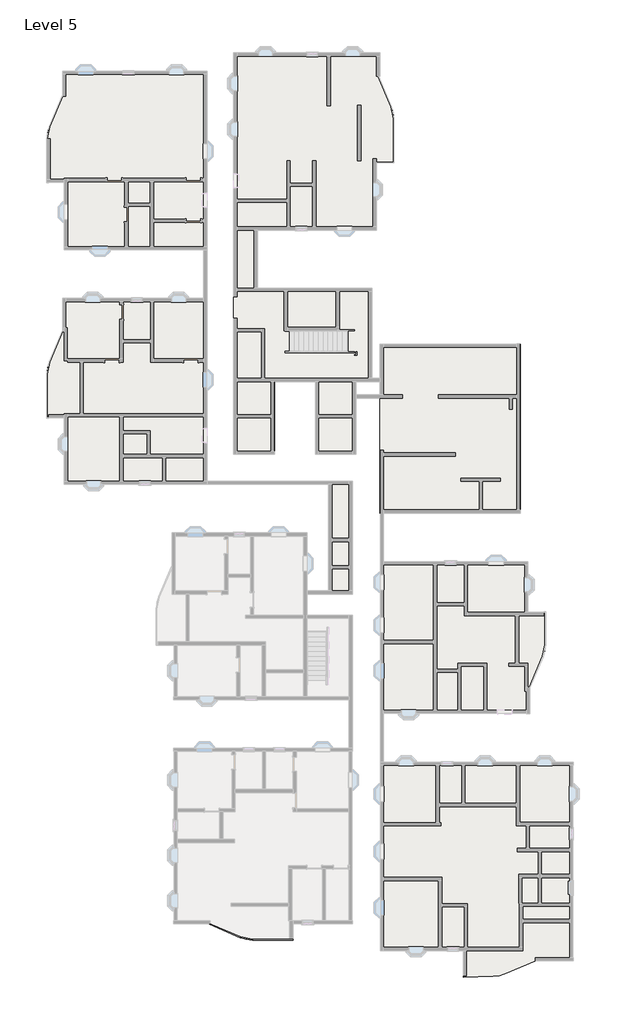
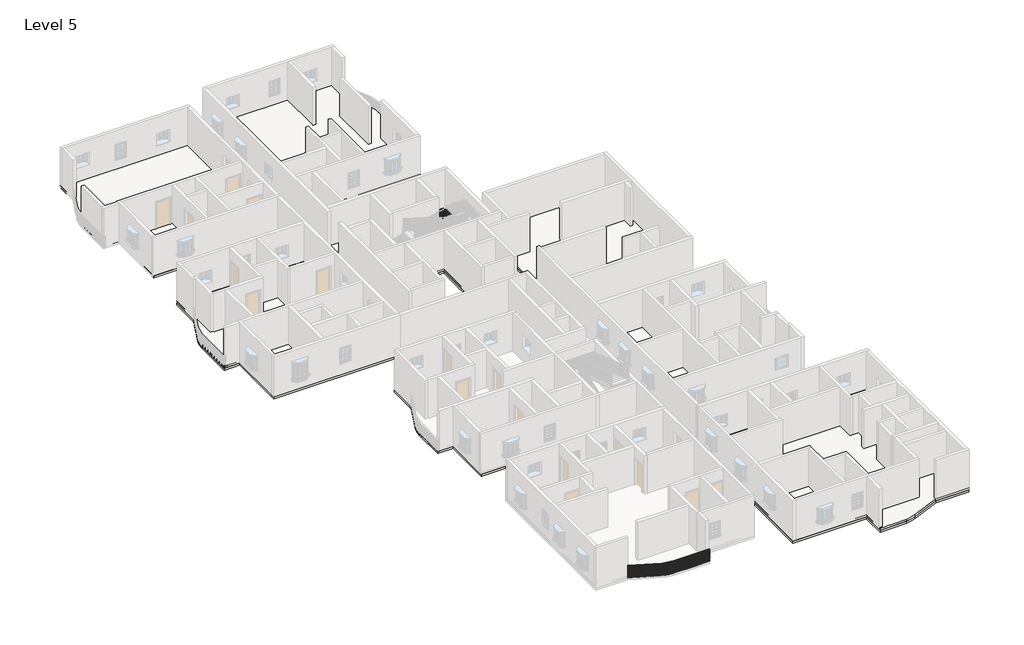
# One storey, part 5 of 14: 11 roofs, 10 slabs, 1 railing.
"""IFC4 building model written with IfcOpenShell, lengths in millimetres."""

from ifc_helpers import new_model, si_unit, point, frame, frame_2d, origin, place, context, project, spatial, polyline, circle_curve, trimmed, segment, composite_curve, outline, extrude, element, save
from ifc_brep_helpers import plane_surface, cylinder_surface, revolved_surface, advanced_brep

model = new_model("IFC4")

# Units and contexts
model_context = context("Model", 3, world=origin())
ifc_project = project(units=[si_unit("LENGTHUNIT", "METRE", prefix="MILLI")], contexts=[model_context])

# Site, building, storey
site = spatial("IfcSite", under=ifc_project)
building = spatial("IfcBuilding", under=site)
storey = spatial("IfcBuildingStorey", under=building, Name="Level 5", Elevation=12192.0)

# Railing
placement = place(None, origin())
element("IfcRailing", 1, ObjectType="Handrail - Rectangular", at=placement, inside=storey, context=model_context, shape_type="SolidModel", body=[
    advanced_brep(
    [(-10014.8722294, -25076.9923935, 13106.4), (-10014.8722294, -25076.9923935, 13055.6), (-10034.8694485, -25123.6909077, 13055.6), (-10034.8694485, -25123.6909077, 13106.4), (-8065.5370278, -25911.7359335, 13106.4), (-8065.5370278, -25911.7359335, 13055.6), (-8085.5342469, -25958.4344477, 13055.6), (-8085.5342469, -25958.4344477, 13106.4), (-7315.6413127, -26065.5416506, 13055.6), (-7315.6413127, -26065.5416506, 13106.4), (-7315.6413127, -26116.3416506, 13055.6), (-7315.6413127, -26116.3416506, 13106.4), (-4746.0891351, -26065.5416506, 13106.4), (-4746.0891351, -26116.3416506, 13106.4), (-4746.0891351, -26116.3416506, 13055.6), (-4746.0891351, -26065.5416506, 13055.6)],
    [
        (0, 1),
        (1, 2),
        (2, 3),
        (3, 0),
        (0, 4),
        (4, 5),
        (5, 1),
        (5, 6),
        (6, 2),
        (6, 7),
        (7, 3),
        (7, 4),
        (8, 5, circle_curve(frame((-7315.6413127, -24160.5416506, 13055.6), z_axis=(0.0, 0.0, -1.0), x_axis=(-0.3936460446736572, -0.9192620907623599, 0.0)), 1905.0)),
        (4, 9, circle_curve(frame((-7315.6413127, -24160.5416506, 13106.4), z_axis=(0.0, 0.0, 1.0), x_axis=(-0.3936460446736572, -0.9192620907623599, 0.0)), 1905.0)),
        (9, 8),
        (10, 6, circle_curve(frame((-7315.6413127, -24160.5416506, 13055.6), z_axis=(0.0, 0.0, -1.0), x_axis=(-0.3936460446736572, -0.9192620907623599, 0.0)), 1955.8)),
        (8, 10),
        (11, 7, circle_curve(frame((-7315.6413127, -24160.5416506, 13106.4), z_axis=(0.0, 0.0, -1.0), x_axis=(-0.3936460446736572, -0.9192620907623599, 0.0)), 1955.8)),
        (10, 11),
        (11, 9),
        (12, 13),
        (13, 14),
        (14, 15),
        (15, 12),
        (9, 12),
        (15, 8),
        (14, 10),
        (13, 11),
    ],
    [
        plane_surface(frame((-10024.8708389, -25100.3416506, 13106.4), z_axis=(-0.9192620907623597, 0.39364604467365766, 0.0), x_axis=(0.39364604467365766, 0.9192620907623597, 0.0))),
        plane_surface(frame((-10014.8722294, -25076.9923935, 13106.4), z_axis=(0.3936460446736573, 0.9192620907623599, 0.0), x_axis=(0.9192620907623599, -0.3936460446736573, 0.0))),
        plane_surface(frame((-10014.8722294, -25076.9923935, 13055.6), z_axis=(0.0, 0.0, -1.0000000000000002), x_axis=(0.9192620907623599, -0.3936460446736573, 0.0))),
        plane_surface(frame((-10034.8694485, -25123.6909077, 13055.6), z_axis=(-0.39364604467365766, -0.9192620907623597, 0.0), x_axis=(0.9192620907623597, -0.39364604467365766, 0.0))),
        plane_surface(frame((-10034.8694485, -25123.6909077, 13106.4), z_axis=(0.0, 0.0, 1.0), x_axis=(0.9192620907623597, -0.39364604467365766, 0.0))),
        revolved_surface(polyline([(-8065.537027803317, -25911.735933502296, 13106.4), (-8065.537027803317, -25911.735933502296, 13055.6)]), (-7315.6413127, -24160.5416506, 13106.4), (0.0, 0.0, 1.0)),
        plane_surface(frame((-7315.6413127, -24160.5416506, 13055.6), z_axis=(0.0, 0.0, -1.0), x_axis=(-0.3936460446736572, -0.9192620907623599, 0.0))),
        cylinder_surface(frame((-7315.6413127, -24160.5416506, 13106.4), z_axis=(0.0, 0.0, 1.0), x_axis=(-0.3936460446736572, -0.9192620907623599, 0.0)), 1955.8),
        plane_surface(frame((-7315.6413127, -24160.5416506, 13106.4), z_axis=(0.0, 0.0, 1.0), x_axis=(-0.3936460446736572, -0.9192620907623599, 0.0))),
        plane_surface(frame((-4746.0891351, -26090.9416506, 13106.4), z_axis=(1.0, 0.0, 0.0), x_axis=(0.0, 1.0, 0.0))),
        plane_surface(frame((-7315.6413127, -26065.5416506, 13106.4), z_axis=(0.0, 1.0, 0.0), x_axis=(1.0, 0.0, 0.0))),
        plane_surface(frame((-7315.6413127, -26065.5416506, 13055.6), z_axis=(0.0, 0.0, -1.0), x_axis=(1.0, 0.0, 0.0))),
        plane_surface(frame((-7315.6413127, -26116.3416506, 13055.6), z_axis=(0.0, -1.0, 0.0), x_axis=(1.0, 0.0, 0.0))),
        plane_surface(frame((-7315.6413127, -26116.3416506, 13106.4), z_axis=(0.0, 0.0, 1.0), x_axis=(1.0, 0.0, 0.0))),
    ],
    [
        (0, [[1, 2, 3, 4]]),
        (1, [[-1, 5, 6, 7]]),
        (2, [[-2, -7, 8, 9]]),
        (3, [[-3, -9, 10, 11]]),
        (4, [[-4, -11, 12, -5]]),
        (5, [[13, -6, 14, 15]]),
        (6, [[16, -8, -13, 17]]),
        (7, [[18, -10, -16, 19]]),
        (8, [[-14, -12, -18, 20]]),
        (9, [[21, 22, 23, 24]]),
        (10, [[-15, 25, -24, 26]]),
        (11, [[-17, -26, -23, 27]]),
        (12, [[-19, -27, -22, 28]]),
        (13, [[-20, -28, -21, -25]]),
    ],
),
    extrude(outline(polyline([(-4785.1663127, -26100.4666506), (-4785.1663127, -26081.4166506), (-4766.1163127, -26081.4166506), (-4766.1163127, -26100.4666506), (-4785.1663127, -26100.4666506)])), frame((0.0, 0.0, 12192.0), z_axis=(0.0, 0.0, 1.0), x_axis=(1.0, 0.0, 0.0)), (0.0, 0.0, 1.0), 863.6),
    extrude(outline(polyline([(-4886.7663127, -26100.4666506), (-4886.7663127, -26081.4166506), (-4867.7163127, -26081.4166506), (-4867.7163127, -26100.4666506), (-4886.7663127, -26100.4666506)])), frame((0.0, 0.0, 12192.0), z_axis=(0.0, 0.0, 1.0), x_axis=(1.0, 0.0, 0.0)), (0.0, 0.0, 1.0), 863.6),
    extrude(outline(polyline([(-4988.3663127, -26100.4666506), (-4988.3663127, -26081.4166506), (-4969.3163127, -26081.4166506), (-4969.3163127, -26100.4666506), (-4988.3663127, -26100.4666506)])), frame((0.0, 0.0, 12192.0), z_axis=(0.0, 0.0, 1.0), x_axis=(1.0, 0.0, 0.0)), (0.0, 0.0, 1.0), 863.6),
    extrude(outline(polyline([(-5089.9663127, -26100.4666506), (-5089.9663127, -26081.4166506), (-5070.9163127, -26081.4166506), (-5070.9163127, -26100.4666506), (-5089.9663127, -26100.4666506)])), frame((0.0, 0.0, 12192.0), z_axis=(0.0, 0.0, 1.0), x_axis=(1.0, 0.0, 0.0)), (0.0, 0.0, 1.0), 863.6),
    extrude(outline(polyline([(-5191.5663127, -26100.4666506), (-5191.5663127, -26081.4166506), (-5172.5163127, -26081.4166506), (-5172.5163127, -26100.4666506), (-5191.5663127, -26100.4666506)])), frame((0.0, 0.0, 12192.0), z_axis=(0.0, 0.0, 1.0), x_axis=(1.0, 0.0, 0.0)), (0.0, 0.0, 1.0), 863.6),
    extrude(outline(polyline([(-5293.1663127, -26100.4666506), (-5293.1663127, -26081.4166506), (-5274.1163127, -26081.4166506), (-5274.1163127, -26100.4666506), (-5293.1663127, -26100.4666506)])), frame((0.0, 0.0, 12192.0), z_axis=(0.0, 0.0, 1.0), x_axis=(1.0, 0.0, 0.0)), (0.0, 0.0, 1.0), 863.6),
    extrude(outline(polyline([(-5394.7663127, -26100.4666506), (-5394.7663127, -26081.4166506), (-5375.7163127, -26081.4166506), (-5375.7163127, -26100.4666506), (-5394.7663127, -26100.4666506)])), frame((0.0, 0.0, 12192.0), z_axis=(0.0, 0.0, 1.0), x_axis=(1.0, 0.0, 0.0)), (0.0, 0.0, 1.0), 863.6),
    extrude(outline(polyline([(-5496.3663127, -26100.4666506), (-5496.3663127, -26081.4166506), (-5477.3163127, -26081.4166506), (-5477.3163127, -26100.4666506), (-5496.3663127, -26100.4666506)])), frame((0.0, 0.0, 12192.0), z_axis=(0.0, 0.0, 1.0), x_axis=(1.0, 0.0, 0.0)), (0.0, 0.0, 1.0), 863.6),
    extrude(outline(polyline([(-5597.9663127, -26100.4666506), (-5597.9663127, -26081.4166506), (-5578.9163127, -26081.4166506), (-5578.9163127, -26100.4666506), (-5597.9663127, -26100.4666506)])), frame((0.0, 0.0, 12192.0), z_axis=(0.0, 0.0, 1.0), x_axis=(1.0, 0.0, 0.0)), (0.0, 0.0, 1.0), 863.6),
    extrude(outline(polyline([(-5699.5663127, -26100.4666506), (-5699.5663127, -26081.4166506), (-5680.5163127, -26081.4166506), (-5680.5163127, -26100.4666506), (-5699.5663127, -26100.4666506)])), frame((0.0, 0.0, 12192.0), z_axis=(0.0, 0.0, 1.0), x_axis=(1.0, 0.0, 0.0)), (0.0, 0.0, 1.0), 863.6),
    extrude(outline(polyline([(-5801.1663127, -26100.4666506), (-5801.1663127, -26081.4166506), (-5782.1163127, -26081.4166506), (-5782.1163127, -26100.4666506), (-5801.1663127, -26100.4666506)])), frame((0.0, 0.0, 12192.0), z_axis=(0.0, 0.0, 1.0), x_axis=(1.0, 0.0, 0.0)), (0.0, 0.0, 1.0), 863.6),
    extrude(outline(polyline([(-5902.7663127, -26100.4666506), (-5902.7663127, -26081.4166506), (-5883.7163127, -26081.4166506), (-5883.7163127, -26100.4666506), (-5902.7663127, -26100.4666506)])), frame((0.0, 0.0, 12192.0), z_axis=(0.0, 0.0, 1.0), x_axis=(1.0, 0.0, 0.0)), (0.0, 0.0, 1.0), 863.6),
    extrude(outline(polyline([(-6004.3663127, -26100.4666506), (-6004.3663127, -26081.4166506), (-5985.3163127, -26081.4166506), (-5985.3163127, -26100.4666506), (-6004.3663127, -26100.4666506)])), frame((0.0, 0.0, 12192.0), z_axis=(0.0, 0.0, 1.0), x_axis=(1.0, 0.0, 0.0)), (0.0, 0.0, 1.0), 863.6),
    extrude(outline(polyline([(-6105.9663127, -26100.4666506), (-6105.9663127, -26081.4166506), (-6086.9163127, -26081.4166506), (-6086.9163127, -26100.4666506), (-6105.9663127, -26100.4666506)])), frame((0.0, 0.0, 12192.0), z_axis=(0.0, 0.0, 1.0), x_axis=(1.0, 0.0, 0.0)), (0.0, 0.0, 1.0), 863.6),
    extrude(outline(polyline([(-6207.5663127, -26100.4666506), (-6207.5663127, -26081.4166506), (-6188.5163127, -26081.4166506), (-6188.5163127, -26100.4666506), (-6207.5663127, -26100.4666506)])), frame((0.0, 0.0, 12192.0), z_axis=(0.0, 0.0, 1.0), x_axis=(1.0, 0.0, 0.0)), (0.0, 0.0, 1.0), 863.6),
    extrude(outline(polyline([(-6309.1663127, -26100.4666506), (-6309.1663127, -26081.4166506), (-6290.1163127, -26081.4166506), (-6290.1163127, -26100.4666506), (-6309.1663127, -26100.4666506)])), frame((0.0, 0.0, 12192.0), z_axis=(0.0, 0.0, 1.0), x_axis=(1.0, 0.0, 0.0)), (0.0, 0.0, 1.0), 863.6),
    extrude(outline(polyline([(-6410.7663127, -26100.4666506), (-6410.7663127, -26081.4166506), (-6391.7163127, -26081.4166506), (-6391.7163127, -26100.4666506), (-6410.7663127, -26100.4666506)])), frame((0.0, 0.0, 12192.0), z_axis=(0.0, 0.0, 1.0), x_axis=(1.0, 0.0, 0.0)), (0.0, 0.0, 1.0), 863.6),
    extrude(outline(polyline([(-6512.3663127, -26100.4666506), (-6512.3663127, -26081.4166506), (-6493.3163127, -26081.4166506), (-6493.3163127, -26100.4666506), (-6512.3663127, -26100.4666506)])), frame((0.0, 0.0, 12192.0), z_axis=(0.0, 0.0, 1.0), x_axis=(1.0, 0.0, 0.0)), (0.0, 0.0, 1.0), 863.6),
    extrude(outline(polyline([(-6613.9663127, -26100.4666506), (-6613.9663127, -26081.4166506), (-6594.9163127, -26081.4166506), (-6594.9163127, -26100.4666506), (-6613.9663127, -26100.4666506)])), frame((0.0, 0.0, 12192.0), z_axis=(0.0, 0.0, 1.0), x_axis=(1.0, 0.0, 0.0)), (0.0, 0.0, 1.0), 863.6),
    extrude(outline(polyline([(-6715.5663127, -26100.4666506), (-6715.5663127, -26081.4166506), (-6696.5163127, -26081.4166506), (-6696.5163127, -26100.4666506), (-6715.5663127, -26100.4666506)])), frame((0.0, 0.0, 12192.0), z_axis=(0.0, 0.0, 1.0), x_axis=(1.0, 0.0, 0.0)), (0.0, 0.0, 1.0), 863.6),
    extrude(outline(polyline([(-6817.1663127, -26100.4666506), (-6817.1663127, -26081.4166506), (-6798.1163127, -26081.4166506), (-6798.1163127, -26100.4666506), (-6817.1663127, -26100.4666506)])), frame((0.0, 0.0, 12192.0), z_axis=(0.0, 0.0, 1.0), x_axis=(1.0, 0.0, 0.0)), (0.0, 0.0, 1.0), 863.6),
    extrude(outline(polyline([(-6918.7663127, -26100.4666506), (-6918.7663127, -26081.4166506), (-6899.7163127, -26081.4166506), (-6899.7163127, -26100.4666506), (-6918.7663127, -26100.4666506)])), frame((0.0, 0.0, 12192.0), z_axis=(0.0, 0.0, 1.0), x_axis=(1.0, 0.0, 0.0)), (0.0, 0.0, 1.0), 863.6),
    extrude(outline(polyline([(-7020.3663127, -26100.4666506), (-7020.3663127, -26081.4166506), (-7001.3163127, -26081.4166506), (-7001.3163127, -26100.4666506), (-7020.3663127, -26100.4666506)])), frame((0.0, 0.0, 12192.0), z_axis=(0.0, 0.0, 1.0), x_axis=(1.0, 0.0, 0.0)), (0.0, 0.0, 1.0), 863.6),
    extrude(outline(polyline([(-7121.9663127, -26100.4666506), (-7121.9663127, -26081.4166506), (-7102.9163127, -26081.4166506), (-7102.9163127, -26100.4666506), (-7121.9663127, -26100.4666506)])), frame((0.0, 0.0, 12192.0), z_axis=(0.0, 0.0, 1.0), x_axis=(1.0, 0.0, 0.0)), (0.0, 0.0, 1.0), 863.6),
    extrude(outline(polyline([(-7223.5663127, -26100.4666506), (-7223.5663127, -26081.4166506), (-7204.5163127, -26081.4166506), (-7204.5163127, -26100.4666506), (-7223.5663127, -26100.4666506)])), frame((0.0, 0.0, 12192.0), z_axis=(0.0, 0.0, 1.0), x_axis=(1.0, 0.0, 0.0)), (0.0, 0.0, 1.0), 863.6),
    extrude(outline(polyline([(-7395.3185803, -26098.8530973), (-7394.6296262, -26079.8155596), (-7375.5920885, -26080.5045137), (-7376.2810426, -26099.5420514), (-7395.3185803, -26098.8530973)])), frame((0.0, 0.0, 12192.0), z_axis=(0.0, 0.0, 1.0), x_axis=(1.0, 0.0, 0.0)), (0.0, 0.0, 1.0), 863.6),
    extrude(outline(polyline([(-7497.177549, -26091.9774704), (-7495.4880357, -26073.0025384), (-7476.5131037, -26074.6920517), (-7478.2026169, -26093.6669837), (-7497.177549, -26091.9774704)])), frame((0.0, 0.0, 12192.0), z_axis=(0.0, 0.0, 1.0), x_axis=(1.0, 0.0, 0.0)), (0.0, 0.0, 1.0), 863.6),
    extrude(outline(polyline([(-7598.5337632, -26079.7528408), (-7595.8483698, -26060.8930645), (-7576.9885935, -26063.5784579), (-7579.6739869, -26082.4382342), (-7598.5337632, -26079.7528408)])), frame((0.0, 0.0, 12192.0), z_axis=(0.0, 0.0, 1.0), x_axis=(1.0, 0.0, 0.0)), (0.0, 0.0, 1.0), 863.6),
    extrude(outline(polyline([(-7699.1065227, -26062.2130639), (-7695.4326862, -26043.5206744), (-7676.7402967, -26047.1945108), (-7680.4141332, -26065.8869003), (-7699.1065227, -26062.2130639)])), frame((0.0, 0.0, 12192.0), z_axis=(0.0, 0.0, 1.0), x_axis=(1.0, 0.0, 0.0)), (0.0, 0.0, 1.0), 863.6),
    extrude(outline(polyline([(-7798.6172969, -26039.4067149), (-7793.9651918, -26020.9334797), (-7775.4919566, -26025.5855848), (-7780.1440617, -26044.05882), (-7798.6172969, -26039.4067149)])), frame((0.0, 0.0, 12192.0), z_axis=(0.0, 0.0, 1.0), x_axis=(1.0, 0.0, 0.0)), (0.0, 0.0, 1.0), 863.6),
    extrude(outline(polyline([(-7896.7904963, -26011.396955), (-7891.1730064, -25993.1940347), (-7872.9700861, -25998.8115246), (-7878.587576, -26017.0144449), (-7896.7904963, -26011.396955)])), frame((0.0, 0.0, 12192.0), z_axis=(0.0, 0.0, 1.0), x_axis=(1.0, 0.0, 0.0)), (0.0, 0.0, 1.0), 863.6),
    extrude(outline(polyline([(-7993.3542357, -25978.2613554), (-7986.7869183, -25960.379162), (-7968.9047249, -25966.9464794), (-7975.4720423, -25984.8286729), (-7993.3542357, -25978.2613554)])), frame((0.0, 0.0, 12192.0), z_axis=(0.0, 0.0, 1.0), x_axis=(1.0, 0.0, 0.0)), (0.0, 0.0, 1.0), 863.6),
    extrude(outline(polyline([(-8169.4357205, -25905.2369062), (-8161.9367633, -25887.7249634), (-8144.4248205, -25895.2239205), (-8151.9237777, -25912.7358634), (-8169.4357205, -25905.2369062)])), frame((0.0, 0.0, 12192.0), z_axis=(0.0, 0.0, 1.0), x_axis=(1.0, 0.0, 0.0)), (0.0, 0.0, 1.0), 863.6),
    extrude(outline(polyline([(-8262.8327489, -25865.2424681), (-8255.3337918, -25847.7305252), (-8237.8218489, -25855.2294824), (-8245.3208061, -25872.7414252), (-8262.8327489, -25865.2424681)])), frame((0.0, 0.0, 12192.0), z_axis=(0.0, 0.0, 1.0), x_axis=(1.0, 0.0, 0.0)), (0.0, 0.0, 1.0), 863.6),
    extrude(outline(polyline([(-8356.2297773, -25825.2480299), (-8348.7308202, -25807.7360871), (-8331.2188774, -25815.2350443), (-8338.7178345, -25832.7469871), (-8356.2297773, -25825.2480299)])), frame((0.0, 0.0, 12192.0), z_axis=(0.0, 0.0, 1.0), x_axis=(1.0, 0.0, 0.0)), (0.0, 0.0, 1.0), 863.6),
    extrude(outline(polyline([(-8449.6268058, -25785.2535918), (-8442.1278486, -25767.741649), (-8424.6159058, -25775.2406061), (-8432.1148629, -25792.752549), (-8449.6268058, -25785.2535918)])), frame((0.0, 0.0, 12192.0), z_axis=(0.0, 0.0, 1.0), x_axis=(1.0, 0.0, 0.0)), (0.0, 0.0, 1.0), 863.6),
    extrude(outline(polyline([(-8543.0238342, -25745.2591537), (-8535.524877, -25727.7472108), (-8518.0129342, -25735.246168), (-8525.5118914, -25752.7581108), (-8543.0238342, -25745.2591537)])), frame((0.0, 0.0, 12192.0), z_axis=(0.0, 0.0, 1.0), x_axis=(1.0, 0.0, 0.0)), (0.0, 0.0, 1.0), 863.6),
    extrude(outline(polyline([(-8636.4208626, -25705.2647155), (-8628.9219055, -25687.7527727), (-8611.4099626, -25695.2517298), (-8618.9089198, -25712.7636727), (-8636.4208626, -25705.2647155)])), frame((0.0, 0.0, 12192.0), z_axis=(0.0, 0.0, 1.0), x_axis=(1.0, 0.0, 0.0)), (0.0, 0.0, 1.0), 863.6),
    extrude(outline(polyline([(-8729.817891, -25665.2702774), (-8722.3189339, -25647.7583346), (-8704.806991, -25655.2572917), (-8712.3059482, -25672.7692345), (-8729.817891, -25665.2702774)])), frame((0.0, 0.0, 12192.0), z_axis=(0.0, 0.0, 1.0), x_axis=(1.0, 0.0, 0.0)), (0.0, 0.0, 1.0), 863.6),
    extrude(outline(polyline([(-8823.2149194, -25625.2758392), (-8815.7159623, -25607.7638964), (-8798.2040195, -25615.2628536), (-8805.7029766, -25632.7747964), (-8823.2149194, -25625.2758392)])), frame((0.0, 0.0, 12192.0), z_axis=(0.0, 0.0, 1.0), x_axis=(1.0, 0.0, 0.0)), (0.0, 0.0, 1.0), 863.6),
    extrude(outline(polyline([(-8916.6119479, -25585.2814011), (-8909.1129907, -25567.7694583), (-8891.6010479, -25575.2684154), (-8899.100005, -25592.7803583), (-8916.6119479, -25585.2814011)])), frame((0.0, 0.0, 12192.0), z_axis=(0.0, 0.0, 1.0), x_axis=(1.0, 0.0, 0.0)), (0.0, 0.0, 1.0), 863.6),
    extrude(outline(polyline([(-9010.0089763, -25545.286963), (-9002.5100191, -25527.7750201), (-8984.9980763, -25535.2739773), (-8992.4970335, -25552.7859201), (-9010.0089763, -25545.286963)])), frame((0.0, 0.0, 12192.0), z_axis=(0.0, 0.0, 1.0), x_axis=(1.0, 0.0, 0.0)), (0.0, 0.0, 1.0), 863.6),
    extrude(outline(polyline([(-9103.4060047, -25505.2925248), (-9095.9070476, -25487.780582), (-9078.3951047, -25495.2795391), (-9085.8940619, -25512.791482), (-9103.4060047, -25505.2925248)])), frame((0.0, 0.0, 12192.0), z_axis=(0.0, 0.0, 1.0), x_axis=(1.0, 0.0, 0.0)), (0.0, 0.0, 1.0), 863.6),
    extrude(outline(polyline([(-9196.8030331, -25465.2980867), (-9189.304076, -25447.7861439), (-9171.7921332, -25455.285101), (-9179.2910903, -25472.7970438), (-9196.8030331, -25465.2980867)])), frame((0.0, 0.0, 12192.0), z_axis=(0.0, 0.0, 1.0), x_axis=(1.0, 0.0, 0.0)), (0.0, 0.0, 1.0), 863.6),
    extrude(outline(polyline([(-9290.2000616, -25425.3036485), (-9282.7011044, -25407.7917057), (-9265.1891616, -25415.2906629), (-9272.6881187, -25432.8026057), (-9290.2000616, -25425.3036485)])), frame((0.0, 0.0, 12192.0), z_axis=(0.0, 0.0, 1.0), x_axis=(1.0, 0.0, 0.0)), (0.0, 0.0, 1.0), 863.6),
    extrude(outline(polyline([(-9383.59709, -25385.3092104), (-9376.0981328, -25367.7972676), (-9358.58619, -25375.2962247), (-9366.0851471, -25392.8081676), (-9383.59709, -25385.3092104)])), frame((0.0, 0.0, 12192.0), z_axis=(0.0, 0.0, 1.0), x_axis=(1.0, 0.0, 0.0)), (0.0, 0.0, 1.0), 863.6),
    extrude(outline(polyline([(-9476.9941184, -25345.3147723), (-9469.4951612, -25327.8028294), (-9451.9832184, -25335.3017866), (-9459.4821756, -25352.8137294), (-9476.9941184, -25345.3147723)])), frame((0.0, 0.0, 12192.0), z_axis=(0.0, 0.0, 1.0), x_axis=(1.0, 0.0, 0.0)), (0.0, 0.0, 1.0), 863.6),
    extrude(outline(polyline([(-9570.3911468, -25305.3203341), (-9562.8921897, -25287.8083913), (-9545.3802468, -25295.3073485), (-9552.879204, -25312.8192913), (-9570.3911468, -25305.3203341)])), frame((0.0, 0.0, 12192.0), z_axis=(0.0, 0.0, 1.0), x_axis=(1.0, 0.0, 0.0)), (0.0, 0.0, 1.0), 863.6),
    extrude(outline(polyline([(-9663.7881752, -25265.325896), (-9656.2892181, -25247.8139532), (-9638.7772753, -25255.3129103), (-9646.2762324, -25272.8248531), (-9663.7881752, -25265.325896)])), frame((0.0, 0.0, 12192.0), z_axis=(0.0, 0.0, 1.0), x_axis=(1.0, 0.0, 0.0)), (0.0, 0.0, 1.0), 863.6),
    extrude(outline(polyline([(-9757.1852037, -25225.3314579), (-9749.6862465, -25207.819515), (-9732.1743037, -25215.3184722), (-9739.6732608, -25232.830415), (-9757.1852037, -25225.3314579)])), frame((0.0, 0.0, 12192.0), z_axis=(0.0, 0.0, 1.0), x_axis=(1.0, 0.0, 0.0)), (0.0, 0.0, 1.0), 863.6),
    extrude(outline(polyline([(-9850.5822321, -25185.3370197), (-9843.0832749, -25167.8250769), (-9825.5713321, -25175.324034), (-9833.0702893, -25192.8359769), (-9850.5822321, -25185.3370197)])), frame((0.0, 0.0, 12192.0), z_axis=(0.0, 0.0, 1.0), x_axis=(1.0, 0.0, 0.0)), (0.0, 0.0, 1.0), 863.6),
    extrude(outline(polyline([(-9943.9792605, -25145.3425816), (-9936.4803034, -25127.8306387), (-9918.9683605, -25135.3295959), (-9926.4673177, -25152.8415387), (-9943.9792605, -25145.3425816)])), frame((0.0, 0.0, 12192.0), z_axis=(0.0, 0.0, 1.0), x_axis=(1.0, 0.0, 0.0)), (0.0, 0.0, 1.0), 863.6),
    extrude(outline(polyline([(-7325.1663127, -26100.4666506), (-7325.1663127, -26081.4166506), (-7306.1163127, -26081.4166506), (-7306.1163127, -26100.4666506), (-7325.1663127, -26100.4666506)])), frame((0.0, 0.0, 12192.0), z_axis=(0.0, 0.0, 1.0), x_axis=(1.0, 0.0, 0.0)), (0.0, 0.0, 1.0), 863.6),
    extrude(outline(polyline([(-8088.0410874, -25940.0916834), (-8080.5421302, -25922.5797406), (-8063.0301874, -25930.0786978), (-8070.5291445, -25947.5906406), (-8088.0410874, -25940.0916834)])), frame((0.0, 0.0, 12192.0), z_axis=(0.0, 0.0, 1.0), x_axis=(1.0, 0.0, 0.0)), (0.0, 0.0, 1.0), 863.6),
    extrude(outline(polyline([(-4765.1391351, -26100.4666506), (-4765.1391351, -26081.4166506), (-4746.0891351, -26081.4166506), (-4746.0891351, -26100.4666506), (-4765.1391351, -26100.4666506)])), frame((0.0, 0.0, 12192.0), z_axis=(0.0, 0.0, 1.0), x_axis=(1.0, 0.0, 0.0)), (0.0, 0.0, 1.0), 863.6),
    extrude(outline(polyline([(-10028.6203175, -25109.097622), (-10021.1213604, -25091.5856792), (-10003.6094175, -25099.0846363), (-10011.1083747, -25116.5965792), (-10028.6203175, -25109.097622)])), frame((0.0, 0.0, 12192.0), z_axis=(0.0, 0.0, 1.0), x_axis=(1.0, 0.0, 0.0)), (0.0, 0.0, 1.0), 863.6),
])

# Roofs
element("IfcRoof", 2, ObjectType="Generic - 12\"", at=placement, inside=storey, context=model_context, shape_type="SweptSolid", body=[
    extrude(outline(composite_curve([segment(polyline([(6070.4380523, -26783.9042694), (812.6380523, -26783.9042694), (812.6380523, -14845.9042694), (13017.3380523, -14845.9042694), (13017.3380523, -27431.6042694), (10660.5280667, -27431.6042694), (8711.1928652, -28266.3478094)]), True, "CONTINUOUS"), segment(trimmed(circle_curve(frame_2d((7951.2985405, -26491.8042694)), 1930.4), [point((8711.1928652, -28266.3478094))], [point((7953.0959373, -28422.2034326))], False, "CARTESIAN"), True, "CONTINUOUS"), segment(polyline([(7953.0959373, -28422.2034326), (6070.4380523, -28487.9472947), (6070.4380523, -26783.9042694)]), True, "CONTINUOUS")], self_intersect=False)), frame((0.0, 0.0, 12192.0), z_axis=(0.0, 0.0, 1.0), x_axis=(1.0, 0.0, 0.0)), (0.0, 0.0, 1.0), 152.4),
])
element("IfcRoof", 3, ObjectType="Generic - 12\"", at=placement, inside=storey, context=model_context, shape_type="SweptSolid", body=[
    extrude(outline(composite_curve([segment(polyline([(10274.1380523, -11759.8042694), (803.8108649, -11759.8042694), (803.8108649, -2133.2042694), (10159.8380523, -2133.2042694), (10159.8380523, -5352.6542694), (11264.7380523, -5352.6542694), (11264.7380523, -7397.5810633)]), True, "CONTINUOUS"), segment(trimmed(circle_curve(frame_2d((9334.3380523, -7397.5810633)), 1930.4), [point((11264.7380523, -7397.5810633))], [point((11108.8815923, -8157.475388))], False, "CARTESIAN"), True, "CONTINUOUS"), segment(polyline([(11108.8815923, -8157.475388), (10274.1380523, -10106.8105895), (10274.1380523, -11759.8042694)]), True, "CONTINUOUS")], self_intersect=False)), frame((0.0, 0.0, 12192.0), z_axis=(0.0, 0.0, 1.0), x_axis=(1.0, 0.0, 0.0)), (0.0, 0.0, 1.0), 152.4),
])
element("IfcRoof", 4, ObjectType="Generic - 12\"", at=placement, inside=storey, context=model_context, shape_type="SweptSolid", body=[
    extrude(outline(polyline([(-2472.7891351, 2953.9583494), (-961.4891351, 2953.9583494), (-961.4891351, -4202.4916506), (-2472.7891351, -4202.4916506), (-2472.7891351, 2953.9583494)])), frame((0.0, 0.0, 12192.0), z_axis=(0.0, 0.0, 1.0), x_axis=(1.0, 0.0, 0.0)), (0.0, 0.0, 1.0), 152.4),
])
element("IfcRoof", 5, ObjectType="Generic - 12\"", at=placement, inside=storey, context=model_context, shape_type="SweptSolid", body=[
    extrude(outline(composite_curve([segment(polyline([(-10194.3891351, 2750.7583494), (-19236.7891351, 2750.7583494), (-19236.7891351, 6979.8583494), (-20341.6891351, 6979.8583494), (-20341.6891351, 9746.7948172)]), True, "CONTINUOUS"), segment(trimmed(circle_curve(frame_2d((-18411.2891351, 9746.7948172)), 1930.4), [point((-20341.6891351, 9746.7948172))], [point((-20185.8326751, 10506.6891419))], False, "CARTESIAN"), True, "CONTINUOUS"), segment(polyline([(-20185.8326751, 10506.6891419), (-19351.0891351, 12456.0243434), (-19351.0891351, 14536.3583494), (-10194.3891351, 14536.3583494), (-10194.3891351, 2750.7583494)]), True, "CONTINUOUS")], self_intersect=False)), frame((0.0, 0.0, 12192.0), z_axis=(0.0, 0.0, 1.0), x_axis=(1.0, 0.0, 0.0)), (0.0, 0.0, 1.0), 152.4),
])
element("IfcRoof", 6, ObjectType="Generic - 12\"", at=placement, inside=storey, context=model_context, shape_type="SweptSolid", body=[
    extrude(outline(polyline([(-8492.5891351, 9478.4949943), (-5914.4891351, 9478.4949943), (-5914.4891351, 4665.1949943), (-8492.5891351, 4665.1949943), (-8492.5891351, 9478.4949943)])), frame((0.0, 0.0, 12192.0), z_axis=(0.0, 0.0, 1.0), x_axis=(1.0, 0.0, 0.0)), (0.0, 0.0, 1.0), 152.4),
])
element("IfcRoof", 7, ObjectType="Generic - 12\"", at=placement, inside=storey, context=model_context, shape_type="SweptSolid", body=[
    extrude(outline(polyline([(-3310.9891351, 9478.4949943), (-745.5891351, 9478.4949943), (-745.5891351, 4652.4949943), (-3310.9891351, 4652.4949943), (-3310.9891351, 9478.4949943)])), frame((0.0, 0.0, 12192.0), z_axis=(0.0, 0.0, 1.0), x_axis=(1.0, 0.0, 0.0)), (0.0, 0.0, 1.0), 152.4),
])
element("IfcRoof", 8, ObjectType="Generic - 12\"", at=placement, inside=storey, context=model_context, shape_type="SweptSolid", body=[
    extrude(outline(polyline([(-8492.5891351, 19078.3215905), (-6993.9891351, 19078.3215905), (-6993.9891351, 14988.9215905), (-8492.5891351, 14988.9215905), (-8492.5891351, 19078.3215905)])), frame((0.0, 0.0, 12192.0), z_axis=(0.0, 0.0, 1.0), x_axis=(1.0, 0.0, 0.0)), (0.0, 0.0, 1.0), 152.4),
])
element("IfcRoof", 9, ObjectType="Generic - 12\"", at=placement, inside=storey, context=model_context, shape_type="SweptSolid", body=[
    extrude(outline(polyline([(-8492.5891351, 15192.1215905), (257.7108649, 15192.1215905), (257.7108649, 9275.2949943), (-8492.5891351, 9275.2949943), (-8492.5891351, 15192.1215905)])), frame((0.0, 0.0, 12192.0), z_axis=(0.0, 0.0, 1.0), x_axis=(1.0, 0.0, 0.0)), (0.0, 0.0, 1.0), 152.4),
])
element("IfcRoof", 10, ObjectType="Generic - 12\"", at=placement, inside=storey, context=model_context, shape_type="SweptSolid", body=[
    extrude(outline(polyline([(793.5880523, 11646.2957306), (9677.2380523, 11646.2957306), (9677.2380523, 940.1957306), (793.5880523, 940.1957306), (793.5880523, 11646.2957306)])), frame((0.0, 0.0, 12192.0), z_axis=(0.0, 0.0, 1.0), x_axis=(1.0, 0.0, 0.0)), (0.0, 0.0, 1.0), 152.4),
])
element("IfcRoof", 11, ObjectType="Generic - 12\"", at=placement, inside=storey, context=model_context, shape_type="SweptSolid", body=[
    extrude(outline(composite_curve([segment(polyline([(-8492.5891351, 18875.1215905), (-8492.5891351, 30101.9215905), (664.1108649, 30101.9215905), (664.1108649, 28631.1875845), (1498.8544049, 26681.8523829)]), True, "CONTINUOUS"), segment(trimmed(circle_curve(frame_2d((-275.6891351, 25921.9580583)), 1930.4), [point((1498.8544049, 26681.8523829))], [point((1654.7108649, 25921.9580583))], False, "CARTESIAN"), True, "CONTINUOUS"), segment(polyline([(1654.7108649, 25921.9580583), (1654.7108649, 23155.0215905), (549.8108649, 23155.0215905), (549.8108649, 18875.1215905), (-8492.5891351, 18875.1215905)]), True, "CONTINUOUS")], self_intersect=False)), frame((0.0, 0.0, 12192.0), z_axis=(0.0, 0.0, 1.0), x_axis=(1.0, 0.0, 0.0)), (0.0, 0.0, 1.0), 152.4),
])
element("IfcRoof", 12, ObjectType="Generic - 12\"", at=placement, inside=storey, context=model_context, shape_type="SweptSolid", body=[
    extrude(outline(composite_curve([segment(polyline([(-10194.3891351, 17609.7583494), (-19236.7891351, 17609.7583494), (-19236.7891351, 21889.6583494), (-20341.6891351, 21889.6583494), (-20341.6891351, 24656.5948172)]), True, "CONTINUOUS"), segment(trimmed(circle_curve(frame_2d((-18411.2891351, 24656.5948172)), 1930.4), [point((-20341.6891351, 24656.5948172))], [point((-20185.8326751, 25416.4891419))], False, "CARTESIAN"), True, "CONTINUOUS"), segment(polyline([(-20185.8326751, 25416.4891419), (-19351.0891351, 27365.8243434), (-19351.0891351, 28950.8583494), (-10194.3891351, 28950.8583494), (-10194.3891351, 17609.7583494)]), True, "CONTINUOUS")], self_intersect=False)), frame((0.0, 0.0, 12192.0), z_axis=(0.0, 0.0, 1.0), x_axis=(1.0, 0.0, 0.0)), (0.0, 0.0, 1.0), 152.4),
])

# Slabs
element("IfcSlab", 13, ObjectType="Generic - 12\"", at=placement, inside=storey, context=model_context, shape_type="SweptSolid", body=[
    extrude(outline(composite_curve([segment(polyline([(13017.3380523, -27431.6042694), (10660.5280667, -27431.6042694), (8711.1928652, -28266.3478094)]), True, "CONTINUOUS"), segment(trimmed(circle_curve(frame_2d((7951.2985405, -26491.8042694)), 1930.4), [point((8711.1928652, -28266.3478094))], [point((7953.0959373, -28422.2034326))], False, "CARTESIAN"), True, "CONTINUOUS"), segment(polyline([(7953.0959373, -28422.2034326), (6070.4380523, -28487.9472947), (6070.4380523, -26783.9042694), (812.6380523, -26783.9042694), (812.6380523, -14845.9042694), (13017.3380523, -14845.9042694), (13017.3380523, -27431.6042694)]), True, "CONTINUOUS")], self_intersect=False)), frame((0.0, 0.0, 12039.6), z_axis=(0.0, 0.0, 1.0), x_axis=(1.0, 0.0, 0.0)), (0.0, 0.0, 1.0), 152.4),
])
element("IfcSlab", 14, ObjectType="Generic - 12\"", at=placement, inside=storey, context=model_context, shape_type="SweptSolid", body=[
    extrude(outline(composite_curve([segment(polyline([(10274.1380523, -11759.8042694), (803.8108649, -11759.8042694), (803.8108649, -2133.2042694), (10159.8380523, -2133.2042694), (10159.8380523, -5352.6542694), (11264.7380523, -5352.6542694), (11264.7380523, -7397.5810633)]), True, "CONTINUOUS"), segment(trimmed(circle_curve(frame_2d((9334.3380523, -7397.5810633)), 1930.4), [point((11264.7380523, -7397.5810633))], [point((11108.8815923, -8157.475388))], False, "CARTESIAN"), True, "CONTINUOUS"), segment(polyline([(11108.8815923, -8157.475388), (10274.1380523, -10106.8105895), (10274.1380523, -11759.8042694)]), True, "CONTINUOUS")], self_intersect=False)), frame((0.0, 0.0, 12039.6), z_axis=(0.0, 0.0, 1.0), x_axis=(1.0, 0.0, 0.0)), (0.0, 0.0, 1.0), 152.4),
])
element("IfcSlab", 15, ObjectType="Generic - 12\"", at=placement, inside=storey, context=model_context, shape_type="SweptSolid", body=[
    extrude(outline(composite_curve([segment(polyline([(-974.1891351, -10889.0416506), (-12290.487215, -10889.0416506), (-12290.487215, -7421.9416506), (-13395.387215, -7421.9416506), (-13395.387215, -5140.4900045)]), True, "CONTINUOUS"), segment(trimmed(circle_curve(frame_2d((-11464.987215, -5140.4900045)), 1930.4), [point((-13395.387215, -5140.4900045))], [point((-13239.530755, -4380.5956799))], False, "CARTESIAN"), True, "CONTINUOUS"), segment(polyline([(-13239.530755, -4380.5956799), (-12404.787215, -2431.2604783), (-12404.787215, -322.6416506), (-3857.687215, -322.6416506), (-3857.687215, -5523.2916506), (-974.1891351, -5523.2916506), (-974.1891351, -10889.0416506)]), True, "CONTINUOUS")], self_intersect=False)), frame((0.0, 0.0, 12039.6), z_axis=(0.0, 0.0, 1.0), x_axis=(1.0, 0.0, 0.0)), (0.0, 0.0, 1.0), 152.4),
])
element("IfcSlab", 16, ObjectType="Generic - 12\"", at=placement, inside=storey, context=model_context, shape_type="SweptSolid", body=[
    extrude(outline(composite_curve([segment(polyline([(-20341.6891351, 6979.8583494), (-20341.6891351, 9746.7948172)]), True, "CONTINUOUS"), segment(trimmed(circle_curve(frame_2d((-18411.2891351, 9746.7948172)), 1930.4), [point((-20341.6891351, 9746.7948172))], [point((-20185.8326751, 10506.6891419))], False, "CARTESIAN"), True, "CONTINUOUS"), segment(polyline([(-20185.8326751, 10506.6891419), (-19351.0891351, 12456.0243434), (-19351.0891351, 14536.3583494), (-10194.3891351, 14536.3583494), (-10194.3891351, 2750.7583494), (-19236.7891351, 2750.7583494), (-19236.7891351, 6979.8583494), (-20341.6891351, 6979.8583494)]), True, "CONTINUOUS")], self_intersect=False)), frame((0.0, 0.0, 12039.6), z_axis=(0.0, 0.0, 1.0), x_axis=(1.0, 0.0, 0.0)), (0.0, 0.0, 1.0), 152.4),
])
element("IfcSlab", 17, ObjectType="Generic - 12\"", at=placement, inside=storey, context=model_context, shape_type="SweptSolid", body=[
    extrude(outline(polyline([(257.7108649, 15192.1215905), (257.7108649, 9275.2949943), (-8492.5891351, 9275.2949943), (-8492.5891351, 15192.1215905), (257.7108649, 15192.1215905)])), frame((0.0, 0.0, 12039.6), z_axis=(0.0, 0.0, 1.0), x_axis=(1.0, 0.0, 0.0)), (0.0, 0.0, 1.0), 152.4),
])
element("IfcSlab", 18, ObjectType="Generic - 12\"", at=placement, inside=storey, context=model_context, shape_type="SweptSolid", body=[
    extrude(outline(polyline([(9677.2380523, 11646.2957306), (9677.2380523, 940.1957306), (793.5880523, 940.1957306), (793.5880523, 11646.2957306), (9677.2380523, 11646.2957306)])), frame((0.0, 0.0, 12039.6), z_axis=(0.0, 0.0, 1.0), x_axis=(1.0, 0.0, 0.0)), (0.0, 0.0, 1.0), 152.4),
])
element("IfcSlab", 19, ObjectType="Generic - 12\"", at=placement, inside=storey, context=model_context, shape_type="SweptSolid", body=[
    extrude(outline(polyline([(-5914.4891351, 9478.4949943), (-5914.4891351, 4665.1949943), (-8492.5891351, 4665.1949943), (-8492.5891351, 9478.4949943), (-5914.4891351, 9478.4949943)])), frame((0.0, 0.0, 12039.6), z_axis=(0.0, 0.0, 1.0), x_axis=(1.0, 0.0, 0.0)), (0.0, 0.0, 1.0), 152.4),
])
element("IfcSlab", 20, ObjectType="Generic - 12\"", at=placement, inside=storey, context=model_context, shape_type="SweptSolid", body=[
    extrude(outline(polyline([(-745.5891351, 9478.4949943), (-745.5891351, 4652.4949943), (-3310.9891351, 4652.4949943), (-3310.9891351, 9478.4949943), (-745.5891351, 9478.4949943)])), frame((0.0, 0.0, 12039.6), z_axis=(0.0, 0.0, 1.0), x_axis=(1.0, 0.0, 0.0)), (0.0, 0.0, 1.0), 152.4),
])
element("IfcSlab", 21, ObjectType="Generic - 12\"", at=placement, inside=storey, context=model_context, shape_type="SweptSolid", body=[
    extrude(outline(polyline([(-961.4891351, 2953.9583494), (-961.4891351, -4202.4916506), (-2472.7891351, -4202.4916506), (-2472.7891351, 2953.9583494), (-961.4891351, 2953.9583494)])), frame((0.0, 0.0, 12039.6), z_axis=(0.0, 0.0, 1.0), x_axis=(1.0, 0.0, 0.0)), (0.0, 0.0, 1.0), 152.4),
])
element("IfcSlab", 22, ObjectType="Generic - 12\"", at=placement, inside=storey, context=model_context, shape_type="SweptSolid", body=[
    extrude(outline(polyline([(-961.4891351, 2953.9583494), (-961.4891351, -4202.4916506), (-2472.7891351, -4202.4916506), (-2472.7891351, 2953.9583494), (-961.4891351, 2953.9583494)])), frame((0.0, 0.0, 12039.6), z_axis=(0.0, 0.0, 1.0), x_axis=(1.0, 0.0, 0.0)), (0.0, 0.0, 1.0), 152.4),
])

save(model, "model.ifc")

# Revit data of these elements
# Type "Handrail - Rectangular"
#   Assembly Code = "C2010400"
#   built-in parameter 1008612 = 0.0416667 (stored number, unit not read)
#   built-in parameter 1008611 = 0.0416667 (stored number, unit not read)
#   built-in parameter 1008609 = 0.333333 (stored number, unit not read)
#   built-in parameter 1008604 = 0.166667 (stored number, unit not read)
#   built-in parameter 1008603 = 0.166667 (stored number, unit not read)
#   Railing Height = 3' - 0"
#   built-in parameter 1008630 = 2
#   built-in parameter 1008610 = 2
#   built-in parameter 1008618 = Baluster - Square : 3/4"
# Type "Generic - 12\""
#   Assembly Code = "B1020"
#   Layers, outside or top first: 0' - 6" no material (function 1)
# Type "Generic - 12\""
#   Assembly Code = "B1010"
#   Function = 0
#   Layers, outside or top first: 0' - 6" no material (function 1)
# Element 1 (IfcRailing, "Handrail - Rectangular")
#   Phase Created = New Construction
# Elements 2, 3, 4, 5, 6, 7, 8, 9, 12 (IfcRoof, "Generic - 12\"")
#   built-in parameter 1001705 = 40.5 (stored number, unit not read)
#   built-in parameter 1001710 = 33615
#   Phase Created = New Construction
#   Materials on its faces: "Default Roof"
# Element 10 (IfcRoof, "Generic - 12\"")
#   built-in parameter 1001705 = 40.5 (stored number, unit not read)
#   built-in parameter 1001710 = 33615
#   Phase Created = New Construction
#   Materials on its faces: "Default Roof", "Carpet (1)"
# Element 11 (IfcRoof, "Generic - 12\"")
#   built-in parameter 1001705 = 40.5 (stored number, unit not read)
#   built-in parameter 1001710 = 33615
#   Phase Created = New Construction
#   Materials on its faces: "Default Roof", "Wood - Stained"
# Elements 13, 15, 17, 19, 20, 21, 22 (IfcSlab, "Generic - 12\"")
#   Height Offset From Level = 0' - 0"
#   Phase Created = New Construction
#   Materials on its faces: "Default Floor"
# Element 14 (IfcSlab, "Generic - 12\"")
#   Height Offset From Level = 0' - 0"
#   Phase Created = New Construction
#   Materials on its faces: "Default Floor", "Wood - Stained"
# Element 16 (IfcSlab, "Generic - 12\"")
#   built-in parameter 1001955 = -1.5708 (stored number, unit not read)
#   Height Offset From Level = 0' - 0"
#   Phase Created = New Construction
#   Materials on its faces: "Default Floor"
# Element 18 (IfcSlab, "Generic - 12\"")
#   Height Offset From Level = 0' - 0"
#   Phase Created = New Construction
#   Materials on its faces: "Default Floor", "Carpet (1)"
# Materials
#   "Default Roof": colour RGB 88 101 114, transparency 0, Cost = 0
#   "Carpet (1)": class "Carpet", colour RGB 124 80 67, transparency 0, Description = "Interior finish", Cost = 0
#   "Wood - Stained": class "Wood", colour RGB 224 178 126, transparency 0, Cost = 0
#   "Default Floor": colour RGB 128 128 128, transparency 0, Cost = 0
